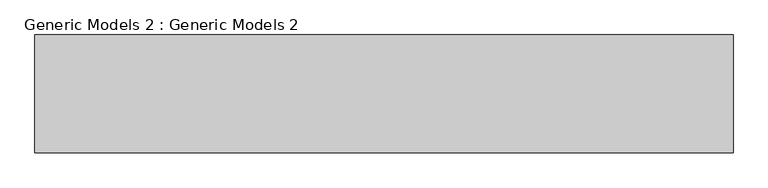
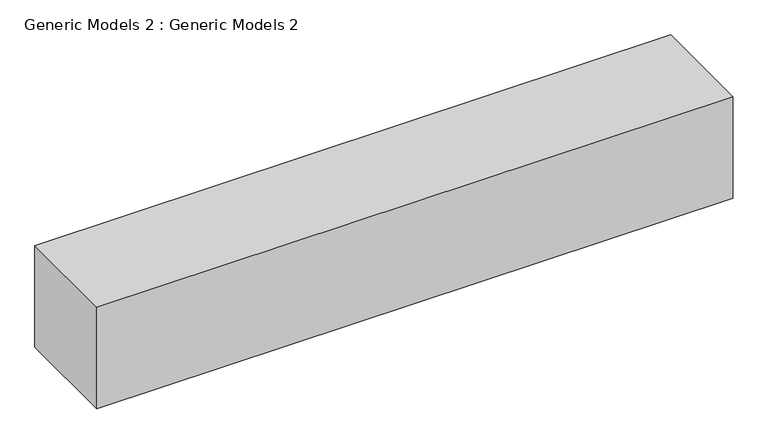
"""IFC4 building model written with IfcOpenShell, lengths in millimetres: proxy geometry, Generic Models 2 : Generic Models 2."""

from ifc_helpers import new_model, si_unit, frame, origin, place, context, project, spatial, polyline, outline, extrude, source, transform, mapped, element, save


def generic_models_2_generic_models_2_050452ab(model_context):
    return source(origin(), model_context, "Body", "SweptSolid", [
        extrude(outline(polyline([(-15380.268705, -4901.1027976), (-12675.168705, -4901.1027976), (-12675.168705, -5358.3027976), (-15380.268705, -5358.3027976), (-15380.268705, -4901.1027976)])), frame((0.0, 0.0, 685.8), z_axis=(0.0, 0.0, 1.0), x_axis=(1.0, 0.0, 0.0)), (0.0, 0.0, 1.0), 457.2),
    ])


if __name__ == "__main__":
    model = new_model("IFC4")
    model_context = context("Model", 3, world=origin())
    ifc_project = project(units=[si_unit("LENGTHUNIT", "METRE", prefix="MILLI")], contexts=[model_context])
    site = spatial("IfcSite", under=ifc_project)
    building = spatial("IfcBuilding", under=site)
    placement = place(None, origin())
    generic_models_2_generic_models_2_shape = generic_models_2_generic_models_2_050452ab(model_context)
    element("IfcBuildingElementProxy", 1, Name="Generic Models 2 : Generic Models 2", ObjectType="Generic Models 2 : Generic Models 2", at=placement, inside=building, context=model_context, shape_type="MappedRepresentation", body=[
        mapped(generic_models_2_generic_models_2_shape, transform((0.0, 0.0, 0.0), x_axis=(1.0, 0.0, 0.0), y_axis=(0.0, 1.0, 0.0), z_axis=(0.0, 0.0, 1.0))),
    ])
    save(model, "model.ifc")

# Revit data of these elements
# Element 1 (IfcBuildingElementProxy, "Generic Models 2 : Generic Models 2")
#   Materials on its faces: "Gypsum Wall Board"
# Materials
#   "Gypsum Wall Board": class "Generic", colour RGB 228 228 228, transparency 0, Description = "Gypsum Wall Board", Cost = 0
